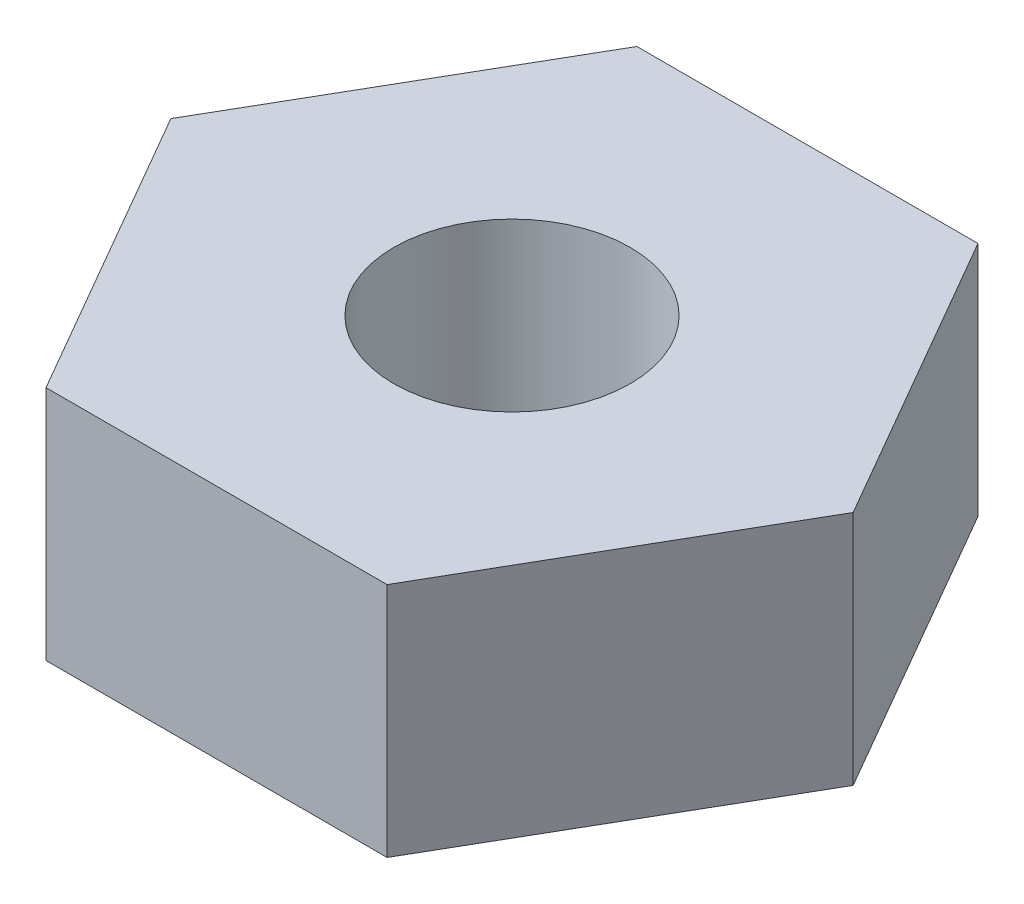
SolidWorks part; units mm, degrees
material "Plain Carbon Steel"
ref_plane "Front Plane" through (0, 0, 0) normal (0, 0, 1) x (1, 0, 0)
ref_plane "Top Plane" through (0, 0, 0) normal (0, 1, 0) x (1, 0, 0)
ref_plane "Right Plane" through (0, 0, 0) normal (1, 0, 0) x (0, 0, -1)
sketch "Hex Nut Profile" plane through (0, 0, 0) normal (0, 1, 0) x (1, 0, 0)
  line L1 (28.8675, 0) -> (14.4338, 25)
  line L2 (14.4338, 25) -> (-14.4338, 25)
  line L3 (-14.4338, 25) -> (-28.8675, 0)
  line L4 (-28.8675, 0) -> (-14.4338, -25)
  line L5 (-14.4338, -25) -> (14.4338, -25)
  line L6 (14.4338, -25) -> (28.8675, 0)
  circle A0 centre (0, 0) radius 25 construction
  circle A1 centre (0, 0) radius 10
  dimension "D2" = 20
  dimension "D1" = 50
extrude "Hex Nut Body" add sketch "Hex Nut Profile" along normal mid plane 20
